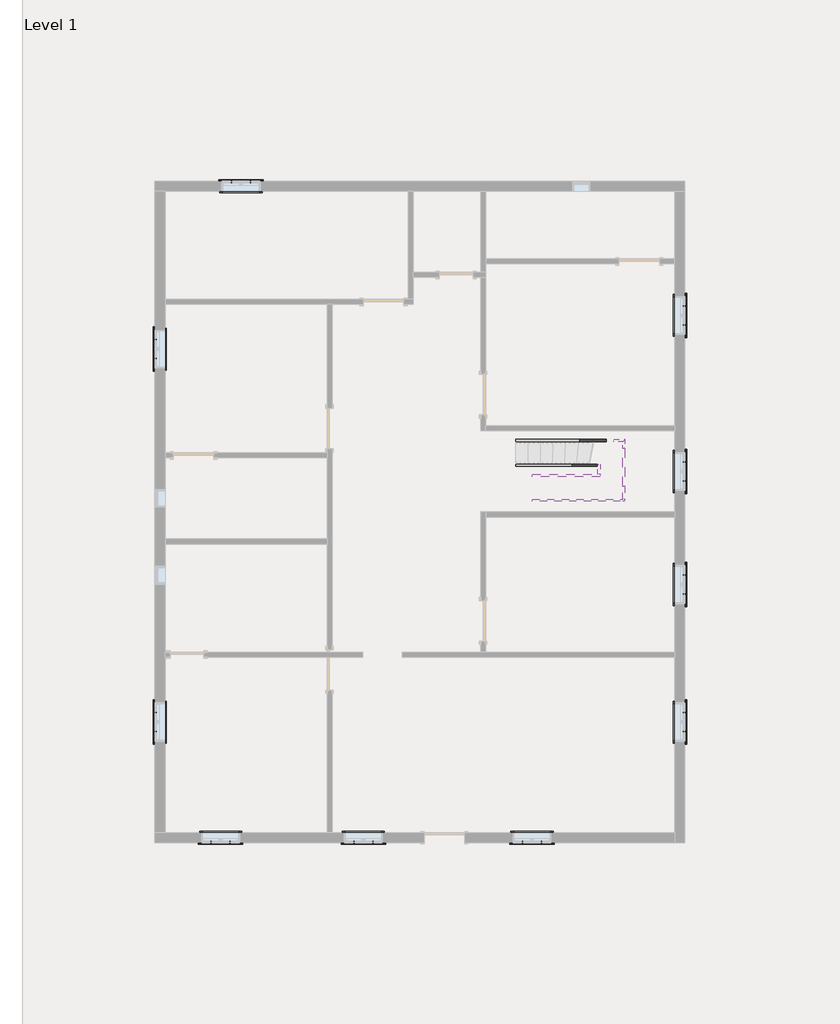
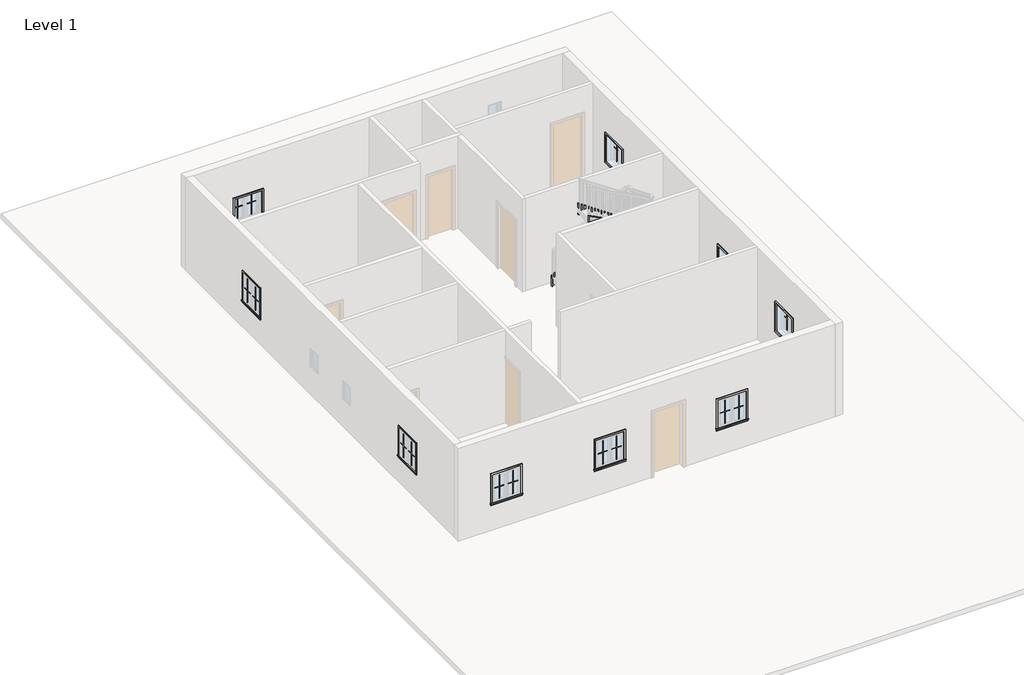
# One storey, part 3 of 3: 40 proxies, 9 members.
"""IFC4 building model written with IfcOpenShell, lengths in millimetres."""

from ifc_helpers import new_model, si_unit, frame, origin, place, context, project, spatial, polyline, outline, extrude, transform, mapped, element, save
from components import muntin_pattern_2x2_muntin_pattern_2x2_b3fe6957, muntin_pattern_2x2_muntin_pattern_2x2_3e0ecaf2, trim_window_exterior_flat_with_sill_41619996, trim_window_interior_flat_picture_frame_51c85655

model = new_model("IFC4")

# Units and contexts
model_context = context("Model", 3, world=origin())
ifc_project = project(units=[si_unit("LENGTHUNIT", "METRE", prefix="MILLI")], contexts=[model_context])

# Site, building, storey
site = spatial("IfcSite", under=ifc_project)
building = spatial("IfcBuilding", under=site)
storey = spatial("IfcBuildingStorey", under=building, Name="Level 1", Elevation=0.0)

# Proxies
placement = place(None, origin())
muntin_pattern_2x2_muntin_pattern_2x2_shape = muntin_pattern_2x2_muntin_pattern_2x2_b3fe6957(model_context)
element("IfcBuildingElementProxy", 1, Name="Muntin Pattern_2x2 : Muntin Pattern_2x2", ObjectType="Muntin Pattern_2x2 : Muntin Pattern_2x2", at=placement, inside=storey, context=model_context, shape_type="MappedRepresentation", body=[
    mapped(muntin_pattern_2x2_muntin_pattern_2x2_shape, transform((-5581.2368007, 9072.452558, 984.25), x_axis=(1.0, 0.0, 0.0), y_axis=(0.0, 1.0, 0.0), z_axis=(0.0, 0.0, 1.0))),
])
element("IfcBuildingElementProxy", 2, Name="Muntin Pattern_2x2 : Muntin Pattern_2x2", ObjectType="Muntin Pattern_2x2 : Muntin Pattern_2x2", at=placement, inside=storey, context=model_context, shape_type="MappedRepresentation", body=[
    mapped(muntin_pattern_2x2_muntin_pattern_2x2_shape, transform((-7300.4993007, 5076.715058, 984.25), x_axis=(0.0, 1.0, 0.0), y_axis=(-1.0, 0.0, 0.0), z_axis=(0.0, 0.0, 1.0))),
])
element("IfcBuildingElementProxy", 3, Name="Muntin Pattern_2x2 : Muntin Pattern_2x2", ObjectType="Muntin Pattern_2x2 : Muntin Pattern_2x2", at=placement, inside=storey, context=model_context, shape_type="MappedRepresentation", body=[
    mapped(muntin_pattern_2x2_muntin_pattern_2x2_shape, transform((4643.8506993, 6267.340058, 984.25), x_axis=(0.0, -1.0, 0.0), y_axis=(1.0, 0.0, 0.0), z_axis=(0.0, 0.0, 1.0))),
])
element("IfcBuildingElementProxy", 4, Name="Muntin Pattern_2x2 : Muntin Pattern_2x2", ObjectType="Muntin Pattern_2x2 : Muntin Pattern_2x2", at=placement, inside=storey, context=model_context, shape_type="MappedRepresentation", body=[
    mapped(muntin_pattern_2x2_muntin_pattern_2x2_shape, transform((4643.8506993, 2743.090058, 984.25), x_axis=(0.0, -1.0, 0.0), y_axis=(1.0, 0.0, 0.0), z_axis=(0.0, 0.0, 1.0))),
])
element("IfcBuildingElementProxy", 5, Name="Muntin Pattern_2x2 : Muntin Pattern_2x2", ObjectType="Muntin Pattern_2x2 : Muntin Pattern_2x2", at=placement, inside=storey, context=model_context, shape_type="MappedRepresentation", body=[
    mapped(muntin_pattern_2x2_muntin_pattern_2x2_shape, transform((4643.8506993, 190.390058, 984.25), x_axis=(0.0, -1.0, 0.0), y_axis=(1.0, 0.0, 0.0), z_axis=(0.0, 0.0, 1.0))),
])
element("IfcBuildingElementProxy", 6, Name="Muntin Pattern_2x2 : Muntin Pattern_2x2", ObjectType="Muntin Pattern_2x2 : Muntin Pattern_2x2", at=placement, inside=storey, context=model_context, shape_type="MappedRepresentation", body=[
    mapped(muntin_pattern_2x2_muntin_pattern_2x2_shape, transform((4643.8506993, -2914.759942, 984.25), x_axis=(0.0, -1.0, 0.0), y_axis=(1.0, 0.0, 0.0), z_axis=(0.0, 0.0, 1.0))),
])
element("IfcBuildingElementProxy", 7, Name="Muntin Pattern_2x2 : Muntin Pattern_2x2", ObjectType="Muntin Pattern_2x2 : Muntin Pattern_2x2", at=placement, inside=storey, context=model_context, shape_type="MappedRepresentation", body=[
    mapped(muntin_pattern_2x2_muntin_pattern_2x2_shape, transform((1419.6381993, -5843.697442, 984.25), x_axis=(-1.0, 0.0, 0.0), y_axis=(0.0, -1.0, 0.0), z_axis=(0.0, 0.0, 1.0))),
])
element("IfcBuildingElementProxy", 8, Name="Muntin Pattern_2x2 : Muntin Pattern_2x2", ObjectType="Muntin Pattern_2x2 : Muntin Pattern_2x2", at=placement, inside=storey, context=model_context, shape_type="MappedRepresentation", body=[
    mapped(muntin_pattern_2x2_muntin_pattern_2x2_shape, transform((-2390.3618007, -5843.697442, 984.25), x_axis=(-1.0, 0.0, 0.0), y_axis=(0.0, -1.0, 0.0), z_axis=(0.0, 0.0, 1.0))),
])
element("IfcBuildingElementProxy", 9, Name="Muntin Pattern_2x2 : Muntin Pattern_2x2", ObjectType="Muntin Pattern_2x2 : Muntin Pattern_2x2", at=placement, inside=storey, context=model_context, shape_type="MappedRepresentation", body=[
    mapped(muntin_pattern_2x2_muntin_pattern_2x2_shape, transform((-5609.8118007, -5843.697442, 984.25), x_axis=(-1.0, 0.0, 0.0), y_axis=(0.0, -1.0, 0.0), z_axis=(0.0, 0.0, 1.0))),
])
element("IfcBuildingElementProxy", 10, Name="Muntin Pattern_2x2 : Muntin Pattern_2x2", ObjectType="Muntin Pattern_2x2 : Muntin Pattern_2x2", at=placement, inside=storey, context=model_context, shape_type="MappedRepresentation", body=[
    mapped(muntin_pattern_2x2_muntin_pattern_2x2_shape, transform((-7300.4993007, -3343.384942, 984.25), x_axis=(0.0, 1.0, 0.0), y_axis=(-1.0, 0.0, 0.0), z_axis=(0.0, 0.0, 1.0))),
])
muntin_pattern_2x2_muntin_pattern_2x2_2_shape = muntin_pattern_2x2_muntin_pattern_2x2_3e0ecaf2(model_context)
element("IfcBuildingElementProxy", 11, Name="Muntin Pattern_2x2 : Muntin Pattern_2x2", ObjectType="Muntin Pattern_2x2 : Muntin Pattern_2x2", at=placement, inside=storey, context=model_context, shape_type="MappedRepresentation", body=[
    mapped(muntin_pattern_2x2_muntin_pattern_2x2_2_shape, transform((-5152.6118007, 9072.452558, 984.25), x_axis=(-1.0, 0.0, 0.0), y_axis=(0.0, -1.0, 0.0), z_axis=(0.0, 0.0, 1.0))),
])
element("IfcBuildingElementProxy", 12, Name="Muntin Pattern_2x2 : Muntin Pattern_2x2", ObjectType="Muntin Pattern_2x2 : Muntin Pattern_2x2", at=placement, inside=storey, context=model_context, shape_type="MappedRepresentation", body=[
    mapped(muntin_pattern_2x2_muntin_pattern_2x2_2_shape, transform((-7300.4993007, 5505.340058, 984.25), x_axis=(0.0, -1.0, 0.0), y_axis=(1.0, 0.0, 0.0), z_axis=(0.0, 0.0, 1.0))),
])
element("IfcBuildingElementProxy", 13, Name="Muntin Pattern_2x2 : Muntin Pattern_2x2", ObjectType="Muntin Pattern_2x2 : Muntin Pattern_2x2", at=placement, inside=storey, context=model_context, shape_type="MappedRepresentation", body=[
    mapped(muntin_pattern_2x2_muntin_pattern_2x2_2_shape, transform((4643.8506993, 5838.715058, 984.25), x_axis=(0.0, 1.0, 0.0), y_axis=(-1.0, 0.0, 0.0), z_axis=(0.0, 0.0, 1.0))),
])
element("IfcBuildingElementProxy", 14, Name="Muntin Pattern_2x2 : Muntin Pattern_2x2", ObjectType="Muntin Pattern_2x2 : Muntin Pattern_2x2", at=placement, inside=storey, context=model_context, shape_type="MappedRepresentation", body=[
    mapped(muntin_pattern_2x2_muntin_pattern_2x2_2_shape, transform((4643.8506993, 2314.465058, 984.25), x_axis=(0.0, 1.0, 0.0), y_axis=(-1.0, 0.0, 0.0), z_axis=(0.0, 0.0, 1.0))),
])
element("IfcBuildingElementProxy", 15, Name="Muntin Pattern_2x2 : Muntin Pattern_2x2", ObjectType="Muntin Pattern_2x2 : Muntin Pattern_2x2", at=placement, inside=storey, context=model_context, shape_type="MappedRepresentation", body=[
    mapped(muntin_pattern_2x2_muntin_pattern_2x2_2_shape, transform((4643.8506993, -238.234942, 984.25), x_axis=(0.0, 1.0, 0.0), y_axis=(-1.0, 0.0, 0.0), z_axis=(0.0, 0.0, 1.0))),
])
element("IfcBuildingElementProxy", 16, Name="Muntin Pattern_2x2 : Muntin Pattern_2x2", ObjectType="Muntin Pattern_2x2 : Muntin Pattern_2x2", at=placement, inside=storey, context=model_context, shape_type="MappedRepresentation", body=[
    mapped(muntin_pattern_2x2_muntin_pattern_2x2_2_shape, transform((4643.8506993, -3343.384942, 984.25), x_axis=(0.0, 1.0, 0.0), y_axis=(-1.0, 0.0, 0.0), z_axis=(0.0, 0.0, 1.0))),
])
element("IfcBuildingElementProxy", 17, Name="Muntin Pattern_2x2 : Muntin Pattern_2x2", ObjectType="Muntin Pattern_2x2 : Muntin Pattern_2x2", at=placement, inside=storey, context=model_context, shape_type="MappedRepresentation", body=[
    mapped(muntin_pattern_2x2_muntin_pattern_2x2_2_shape, transform((991.0131993, -5843.697442, 984.25), x_axis=(1.0, 0.0, 0.0), y_axis=(0.0, 1.0, 0.0), z_axis=(0.0, 0.0, 1.0))),
])
element("IfcBuildingElementProxy", 18, Name="Muntin Pattern_2x2 : Muntin Pattern_2x2", ObjectType="Muntin Pattern_2x2 : Muntin Pattern_2x2", at=placement, inside=storey, context=model_context, shape_type="MappedRepresentation", body=[
    mapped(muntin_pattern_2x2_muntin_pattern_2x2_2_shape, transform((-2818.9868007, -5843.697442, 984.25), x_axis=(1.0, 0.0, 0.0), y_axis=(0.0, 1.0, 0.0), z_axis=(0.0, 0.0, 1.0))),
])
element("IfcBuildingElementProxy", 19, Name="Muntin Pattern_2x2 : Muntin Pattern_2x2", ObjectType="Muntin Pattern_2x2 : Muntin Pattern_2x2", at=placement, inside=storey, context=model_context, shape_type="MappedRepresentation", body=[
    mapped(muntin_pattern_2x2_muntin_pattern_2x2_2_shape, transform((-6038.4368007, -5843.697442, 984.25), x_axis=(1.0, 0.0, 0.0), y_axis=(0.0, 1.0, 0.0), z_axis=(0.0, 0.0, 1.0))),
])
element("IfcBuildingElementProxy", 20, Name="Muntin Pattern_2x2 : Muntin Pattern_2x2", ObjectType="Muntin Pattern_2x2 : Muntin Pattern_2x2", at=placement, inside=storey, context=model_context, shape_type="MappedRepresentation", body=[
    mapped(muntin_pattern_2x2_muntin_pattern_2x2_2_shape, transform((-7300.4993007, -2914.759942, 984.25), x_axis=(0.0, -1.0, 0.0), y_axis=(1.0, 0.0, 0.0), z_axis=(0.0, 0.0, 1.0))),
])
trim_window_exterior_flat_with_sill_shape = trim_window_exterior_flat_with_sill_41619996(model_context)
element("IfcBuildingElementProxy", 21, Name="Trim-Window-Exterior-Flat : with Sill", ObjectType="Trim-Window-Exterior-Flat : with Sill", at=placement, inside=storey, context=model_context, shape_type="MappedRepresentation", body=[
    mapped(trim_window_exterior_flat_with_sill_shape, transform((-5366.9243007, 9081.977558, 1828.8), x_axis=(-1.0, 0.0, 0.0), y_axis=(0.0, 0.0, 1.0), z_axis=(0.0, 1.0, 0.0))),
])
element("IfcBuildingElementProxy", 22, Name="Trim-Window-Exterior-Flat : with Sill", ObjectType="Trim-Window-Exterior-Flat : with Sill", at=placement, inside=storey, context=model_context, shape_type="MappedRepresentation", body=[
    mapped(trim_window_exterior_flat_with_sill_shape, transform((-7310.0243007, 5291.027558, 1828.8), x_axis=(0.0, -1.0, 0.0), y_axis=(0.0, 0.0, 1.0), z_axis=(-1.0, 0.0, 0.0))),
])
element("IfcBuildingElementProxy", 23, Name="Trim-Window-Exterior-Flat : with Sill", ObjectType="Trim-Window-Exterior-Flat : with Sill", at=placement, inside=storey, context=model_context, shape_type="MappedRepresentation", body=[
    mapped(trim_window_exterior_flat_with_sill_shape, transform((4653.3756993, 6053.027558, 1828.8), x_axis=(0.0, 1.0, 0.0), y_axis=(0.0, 0.0, 1.0), z_axis=(1.0, 0.0, 0.0))),
])
element("IfcBuildingElementProxy", 24, Name="Trim-Window-Exterior-Flat : with Sill", ObjectType="Trim-Window-Exterior-Flat : with Sill", at=placement, inside=storey, context=model_context, shape_type="MappedRepresentation", body=[
    mapped(trim_window_exterior_flat_with_sill_shape, transform((4653.3756993, 2528.777558, 1828.8), x_axis=(0.0, 1.0, 0.0), y_axis=(0.0, 0.0, 1.0), z_axis=(1.0, 0.0, 0.0))),
])
element("IfcBuildingElementProxy", 25, Name="Trim-Window-Exterior-Flat : with Sill", ObjectType="Trim-Window-Exterior-Flat : with Sill", at=placement, inside=storey, context=model_context, shape_type="MappedRepresentation", body=[
    mapped(trim_window_exterior_flat_with_sill_shape, transform((4653.3756993, -23.922442, 1828.8), x_axis=(0.0, 1.0, 0.0), y_axis=(0.0, 0.0, 1.0), z_axis=(1.0, 0.0, 0.0))),
])
element("IfcBuildingElementProxy", 26, Name="Trim-Window-Exterior-Flat : with Sill", ObjectType="Trim-Window-Exterior-Flat : with Sill", at=placement, inside=storey, context=model_context, shape_type="MappedRepresentation", body=[
    mapped(trim_window_exterior_flat_with_sill_shape, transform((4653.3756993, -3129.072442, 1828.8), x_axis=(0.0, 1.0, 0.0), y_axis=(0.0, 0.0, 1.0), z_axis=(1.0, 0.0, 0.0))),
])
element("IfcBuildingElementProxy", 27, Name="Trim-Window-Exterior-Flat : with Sill", ObjectType="Trim-Window-Exterior-Flat : with Sill", at=placement, inside=storey, context=model_context, shape_type="MappedRepresentation", body=[
    mapped(trim_window_exterior_flat_with_sill_shape, transform((1205.3256993, -5853.222442, 1828.8), x_axis=(1.0, 0.0, 0.0), y_axis=(0.0, 0.0, 1.0), z_axis=(0.0, -1.0, 0.0))),
])
element("IfcBuildingElementProxy", 28, Name="Trim-Window-Exterior-Flat : with Sill", ObjectType="Trim-Window-Exterior-Flat : with Sill", at=placement, inside=storey, context=model_context, shape_type="MappedRepresentation", body=[
    mapped(trim_window_exterior_flat_with_sill_shape, transform((-2604.6743007, -5853.222442, 1828.8), x_axis=(1.0, 0.0, 0.0), y_axis=(0.0, 0.0, 1.0), z_axis=(0.0, -1.0, 0.0))),
])
element("IfcBuildingElementProxy", 29, Name="Trim-Window-Exterior-Flat : with Sill", ObjectType="Trim-Window-Exterior-Flat : with Sill", at=placement, inside=storey, context=model_context, shape_type="MappedRepresentation", body=[
    mapped(trim_window_exterior_flat_with_sill_shape, transform((-5824.1243007, -5853.222442, 1828.8), x_axis=(1.0, 0.0, 0.0), y_axis=(0.0, 0.0, 1.0), z_axis=(0.0, -1.0, 0.0))),
])
element("IfcBuildingElementProxy", 30, Name="Trim-Window-Exterior-Flat : with Sill", ObjectType="Trim-Window-Exterior-Flat : with Sill", at=placement, inside=storey, context=model_context, shape_type="MappedRepresentation", body=[
    mapped(trim_window_exterior_flat_with_sill_shape, transform((-7310.0243007, -3129.072442, 1828.8), x_axis=(0.0, -1.0, 0.0), y_axis=(0.0, 0.0, 1.0), z_axis=(-1.0, 0.0, 0.0))),
])
trim_window_interior_flat_picture_frame_shape = trim_window_interior_flat_picture_frame_51c85655(model_context)
element("IfcBuildingElementProxy", 31, Name="Trim-Window-Interior-Flat : Picture Frame", ObjectType="Trim-Window-Interior-Flat : Picture Frame", at=placement, inside=storey, context=model_context, shape_type="MappedRepresentation", body=[
    mapped(trim_window_interior_flat_picture_frame_shape, transform((-5366.9243007, 8853.377558, 1828.8), x_axis=(1.0, 0.0, 0.0), y_axis=(0.0, 0.0, 1.0), z_axis=(0.0, -1.0, 0.0))),
])
element("IfcBuildingElementProxy", 32, Name="Trim-Window-Interior-Flat : Picture Frame", ObjectType="Trim-Window-Interior-Flat : Picture Frame", at=placement, inside=storey, context=model_context, shape_type="MappedRepresentation", body=[
    mapped(trim_window_interior_flat_picture_frame_shape, transform((-7081.4243007, 5291.027558, 1828.8), x_axis=(0.0, 1.0, 0.0), y_axis=(0.0, 0.0, 1.0), z_axis=(1.0, 0.0, 0.0))),
])
element("IfcBuildingElementProxy", 33, Name="Trim-Window-Interior-Flat : Picture Frame", ObjectType="Trim-Window-Interior-Flat : Picture Frame", at=placement, inside=storey, context=model_context, shape_type="MappedRepresentation", body=[
    mapped(trim_window_interior_flat_picture_frame_shape, transform((4424.7756993, 6053.027558, 1828.8), x_axis=(0.0, -1.0, 0.0), y_axis=(0.0, 0.0, 1.0), z_axis=(-1.0, 0.0, 0.0))),
])
element("IfcBuildingElementProxy", 34, Name="Trim-Window-Interior-Flat : Picture Frame", ObjectType="Trim-Window-Interior-Flat : Picture Frame", at=placement, inside=storey, context=model_context, shape_type="MappedRepresentation", body=[
    mapped(trim_window_interior_flat_picture_frame_shape, transform((4424.7756993, 2528.777558, 1828.8), x_axis=(0.0, -1.0, 0.0), y_axis=(0.0, 0.0, 1.0), z_axis=(-1.0, 0.0, 0.0))),
])
element("IfcBuildingElementProxy", 35, Name="Trim-Window-Interior-Flat : Picture Frame", ObjectType="Trim-Window-Interior-Flat : Picture Frame", at=placement, inside=storey, context=model_context, shape_type="MappedRepresentation", body=[
    mapped(trim_window_interior_flat_picture_frame_shape, transform((4424.7756993, -23.922442, 1828.8), x_axis=(0.0, -1.0, 0.0), y_axis=(0.0, 0.0, 1.0), z_axis=(-1.0, 0.0, 0.0))),
])
element("IfcBuildingElementProxy", 36, Name="Trim-Window-Interior-Flat : Picture Frame", ObjectType="Trim-Window-Interior-Flat : Picture Frame", at=placement, inside=storey, context=model_context, shape_type="MappedRepresentation", body=[
    mapped(trim_window_interior_flat_picture_frame_shape, transform((4424.7756993, -3129.072442, 1828.8), x_axis=(0.0, -1.0, 0.0), y_axis=(0.0, 0.0, 1.0), z_axis=(-1.0, 0.0, 0.0))),
])
element("IfcBuildingElementProxy", 37, Name="Trim-Window-Interior-Flat : Picture Frame", ObjectType="Trim-Window-Interior-Flat : Picture Frame", at=placement, inside=storey, context=model_context, shape_type="MappedRepresentation", body=[
    mapped(trim_window_interior_flat_picture_frame_shape, transform((1205.3256993, -5624.622442, 1828.8), x_axis=(-1.0, 0.0, 0.0), y_axis=(0.0, 0.0, 1.0), z_axis=(0.0, 1.0, 0.0))),
])
element("IfcBuildingElementProxy", 38, Name="Trim-Window-Interior-Flat : Picture Frame", ObjectType="Trim-Window-Interior-Flat : Picture Frame", at=placement, inside=storey, context=model_context, shape_type="MappedRepresentation", body=[
    mapped(trim_window_interior_flat_picture_frame_shape, transform((-2604.6743007, -5624.622442, 1828.8), x_axis=(-1.0, 0.0, 0.0), y_axis=(0.0, 0.0, 1.0), z_axis=(0.0, 1.0, 0.0))),
])
element("IfcBuildingElementProxy", 39, Name="Trim-Window-Interior-Flat : Picture Frame", ObjectType="Trim-Window-Interior-Flat : Picture Frame", at=placement, inside=storey, context=model_context, shape_type="MappedRepresentation", body=[
    mapped(trim_window_interior_flat_picture_frame_shape, transform((-5824.1243007, -5624.622442, 1828.8), x_axis=(-1.0, 0.0, 0.0), y_axis=(0.0, 0.0, 1.0), z_axis=(0.0, 1.0, 0.0))),
])
element("IfcBuildingElementProxy", 40, Name="Trim-Window-Interior-Flat : Picture Frame", ObjectType="Trim-Window-Interior-Flat : Picture Frame", at=placement, inside=storey, context=model_context, shape_type="MappedRepresentation", body=[
    mapped(trim_window_interior_flat_picture_frame_shape, transform((-7081.4243007, -3129.072442, 1828.8), x_axis=(0.0, 1.0, 0.0), y_axis=(0.0, 0.0, 1.0), z_axis=(1.0, 0.0, 0.0))),
])

# Members
element("IfcMember", 41, ObjectType="Stringer - 2\" Width", at=placement, inside=storey, context=model_context, shape_type="SweptSolid", body=[
    extrude(outline(polyline([(388.4746569, 838.4202681), (37.8072902, 838.4202681), (1297.4160324, 3052.6525996), (1648.0833991, 3052.6525996), (388.4746569, 838.4202681)])), frame((0.0, 3202.4524989, 0.0), z_axis=(0.0, 1.0, 0.0), x_axis=(0.0, 0.0, 1.0)), (0.0, 0.0, 1.0), 50.8),
])
element("IfcMember", 42, ObjectType="Stringer - 2\" Width", at=placement, inside=storey, context=model_context, shape_type="SweptSolid", body=[
    extrude(outline(polyline([(3052.6525996, 3202.4524989), (3052.6525996, 3253.2524989), (3298.782332, 3253.2524989), (3247.982332, 3202.4524989), (3052.6525996, 3202.4524989)])), frame((0.0, 0.0, 1297.4160324), z_axis=(0.0, 0.0, 1.0), x_axis=(1.0, 0.0, 0.0)), (0.0, 0.0, 1.0), 350.6673667),
])
element("IfcMember", 43, ObjectType="Stringer - 2\" Width", at=placement, inside=storey, context=model_context, shape_type="SweptSolid", body=[
    extrude(outline(polyline([(3247.982332, 3202.4524989), (3298.782332, 3253.2524989), (3298.782332, 3048.1586437), (3247.982332, 3048.1586437), (3247.982332, 3202.4524989)])), frame((0.0, 0.0, 1297.4160324), z_axis=(0.0, 0.0, 1.0), x_axis=(1.0, 0.0, 0.0)), (0.0, 0.0, 1.0), 350.6673667),
])
element("IfcMember", 44, ObjectType="Stringer - 2\" Width", at=placement, inside=storey, context=model_context, shape_type="SweptSolid", body=[
    extrude(outline(polyline([(3048.1586437, 1648.0833991), (3048.1586437, 1297.4160324), (2198.376501, 1652.9779505), (2198.376501, 2003.6453172), (3048.1586437, 1648.0833991)])), frame((3247.982332, 0.0, 0.0), z_axis=(1.0, 0.0, 0.0), x_axis=(0.0, 1.0, 0.0)), (0.0, 0.0, 1.0), 50.8),
])
element("IfcMember", 45, ObjectType="Stringer - 2\" Width", at=placement, inside=storey, context=model_context, shape_type="SweptSolid", body=[
    extrude(outline(polyline([(3247.982332, 2198.376501), (3298.782332, 2198.376501), (3298.782332, 1905.9026171), (3247.982332, 1905.9026171), (3247.982332, 2198.376501)])), frame((0.0, 0.0, 1661.9761112), z_axis=(0.0, 0.0, 1.0), x_axis=(1.0, 0.0, 0.0)), (0.0, 0.0, 1.0), 330.4053693),
])
element("IfcMember", 46, ObjectType="Stringer - 2\" Width", at=placement, inside=storey, context=model_context, shape_type="SweptSolid", body=[
    extrude(outline(polyline([(374.0558321, 838.4202681), (11.1163437, 838.4202681), (1207.1401496, 2688.6073911), (1570.0796379, 2688.6073911), (374.0558321, 838.4202681)])), frame((0.0, 2643.077558, 0.0), z_axis=(0.0, 1.0, 0.0), x_axis=(0.0, 0.0, 1.0)), (0.0, 0.0, 1.0), 50.8),
])
element("IfcMember", 47, ObjectType="Stringer - 2\" Width", at=placement, inside=storey, context=model_context, shape_type="SweptSolid", body=[
    extrude(outline(polyline([(2693.877558, 1737.4149577), (2693.877558, 1290.1996268), (2465.277558, 1535.6439445), (2465.277558, 1982.8592754), (2693.877558, 1737.4149577)])), frame((2688.6073911, 0.0, 0.0), z_axis=(1.0, 0.0, 0.0), x_axis=(0.0, 1.0, 0.0)), (0.0, 0.0, 1.0), 50.8),
])
element("IfcMember", 48, ObjectType="Stringer - 2\" Width", at=placement, inside=storey, context=model_context, shape_type="SweptSolid", body=[
    extrude(outline(polyline([(1700.7150039, 2739.4073911), (2070.691358, 2739.4073911), (3121.8229383, 1211.6756993), (2751.8465842, 1211.6756993), (1700.7150039, 2739.4073911)])), frame((0.0, 2414.477558, 0.0), z_axis=(0.0, 1.0, 0.0), x_axis=(0.0, 0.0, 1.0)), (0.0, 0.0, 1.0), 50.8),
])
element("IfcMember", 49, ObjectType="Stringer - 2\" Width", at=placement, inside=storey, context=model_context, shape_type="SweptSolid", body=[
    extrude(outline(polyline([(1687.5814805, 3298.782332), (1965.9410006, 3298.782332), (3052.242202, 1211.6756993), (2721.8368327, 1211.6756993), (1687.5814805, 3198.7868271), (1687.5814805, 3298.782332)])), frame((0.0, 1855.1026171, 0.0), z_axis=(0.0, 1.0, 0.0), x_axis=(0.0, 0.0, 1.0)), (0.0, 0.0, 1.0), 50.8),
])

save(model, "model.ifc")

# Revit data of these elements
# Type "Muntin Pattern_2x2 : Muntin Pattern_2x2"
#   Width [instance default] = 4' - 0"
#   Thickness = 0' - 0 1/2"
#   Height [instance default] = 4' - 0"
#   Distance = 0' - 0 3/4"
#   Interior Material [instance default] = none
#   Exterior Material [instance default] = none
#   Default Elevation = 0
# Type "Trim-Window-Exterior-Flat : with Sill"
#   Trim Width = 0' - 2 1/4"
#   Trim Thickness_Picture Frame = 0' - 1 1/4"
#   Trim Thickness_with Sill = 0' - 0 3/4"
#   Sill Thickness = 0' - 1 1/4"
#   Opening Width [instance default] = 2' - 0"
#   Opening Height [instance default] = 3' - 0"
#   Default Elevation = 4' - 0"
#   Sill = yes
#   Picture Frame = no
#   Trim Material [instance default] = none
# Type "Trim-Window-Interior-Flat : Picture Frame"
#   Trim Thickness_Picture Frame = 0' - 1 1/4"
#   Trim Width = 0' - 2 1/4"
#   Trim Thickness_with Sill = 0' - 0 3/4"
#   Sill Thickness = 0' - 1 1/4"
#   Opening Width [instance default] = 2' - 0"
#   Opening Height [instance default] = 3' - 0"
#   Default Elevation = 4' - 0"
#   Sill = no
#   Picture Frame = yes
#   Trim Material [instance default] = none
# Elements 1, 2, 3, 4, 5, 6, 7, 8, 9, 10, 11, 12, 13, 14, 15, 16, 17, 18, 19, 20 (IfcBuildingElementProxy, "Muntin Pattern_2x2 : Muntin Pattern_2x2")
#   Width = 0' - 11 5/8"
#   Height = 2' - 6 1/2"
#   Interior Material = Wood - Stained
#   Exterior Material = Clad - White
#   Phase Created = New Construction
#   Materials on its faces: "Clad - White", "Wood - Stained"
# Elements 21, 22, 23, 24, 25, 26, 27, 28, 29, 30 (IfcBuildingElementProxy, "Trim-Window-Exterior-Flat : with Sill")
#   Opening Width = 2' - 10"
#   Opening Height = 3' - 0"
#   Trim Material = Clad - White
#   Phase Created = New Construction
#   Materials on its faces: "Clad - White"
# Elements 31, 32, 33, 34, 35, 36, 37, 38, 39, 40 (IfcBuildingElementProxy, "Trim-Window-Interior-Flat : Picture Frame")
#   Opening Width = 2' - 10"
#   Opening Height = 3' - 0"
#   Trim Material = Wood - Stained
#   Phase Created = New Construction
#   Materials on its faces: "Wood - Stained"
# Elements 41, 42, 43, 44, 45, 46, 47, 48, 49 (IfcMember, "Stringer - 2\" Width")
#   Phase Created = New Construction
# Materials
#   "Clad - White": class "Wood", colour RGB 242 242 238, transparency 0, Cost = 0
#   "Wood - Stained": class "Wood", colour RGB 224 178 126, transparency 0, Cost = 0
